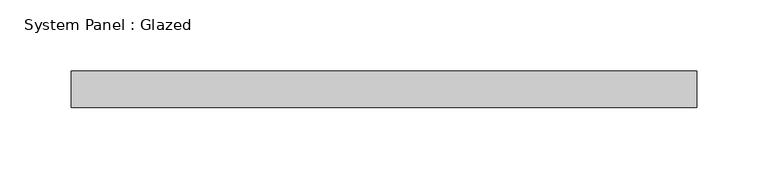
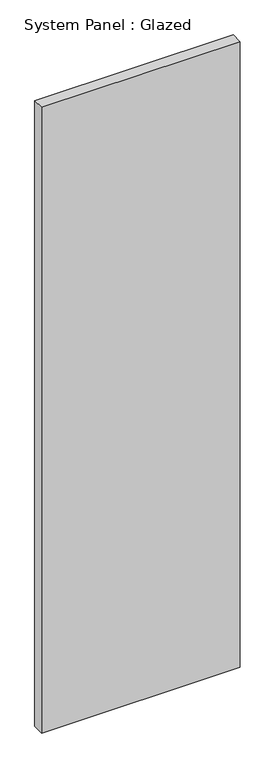
"""IFC4 building model written with IfcOpenShell, lengths in millimetres: plate geometry, System Panel : Glazed."""

from ifc_helpers import new_model, si_unit, origin, origin_with_axes, place, context, project, spatial, polyline, outline, extrude, source, transform, mapped, element, save


def system_panel_glazed_e16a1513(model_context):
    return source(origin(), model_context, "Body", "SweptSolid", [
        extrude(outline(polyline([(219.075, 19.05), (-219.075, 19.05), (-219.075, 44.45), (219.075, 44.45), (219.075, 19.05)])), origin_with_axes(), (0.0, 0.0, 1.0), 1459.1267095),
    ])


if __name__ == "__main__":
    model = new_model("IFC4")
    model_context = context("Model", 3, world=origin())
    ifc_project = project(units=[si_unit("LENGTHUNIT", "METRE", prefix="MILLI")], contexts=[model_context])
    site = spatial("IfcSite", under=ifc_project)
    building = spatial("IfcBuilding", under=site)
    placement = place(None, origin())
    system_panel_glazed_shape = system_panel_glazed_e16a1513(model_context)
    element("IfcPlate", 1, ObjectType="System Panel : Glazed", at=placement, inside=building, context=model_context, shape_type="MappedRepresentation", body=[
        mapped(system_panel_glazed_shape, transform((0.0, 0.0, 0.0), x_axis=(1.0, 0.0, 0.0), y_axis=(0.0, 1.0, 0.0), z_axis=(0.0, 0.0, 1.0))),
    ])
    save(model, "model.ifc")

# Revit data of these elements
# Type "System Panel : Glazed"
#   Construction Type Id = "GSP4R"
#   Analytic Construction = "1/8 in Pilkington single glazing"
#   Visual Light Transmittance = 0.9
#   Solar Heat Gain Coefficient = 0.86
#   Heat Transfer Coefficient (U) = 1.18115 BTU/(h·ft²·°F)
#   Define Thermal Properties by = 1
# Element 1 (IfcPlate, "System Panel : Glazed")
#   Materials on its faces: "Glass"
# Materials
#   "Glass": class "Glass", colour RGB 0 128 192, transparency 0.75, Description = "Soda Lime Glass", Cost = 0
